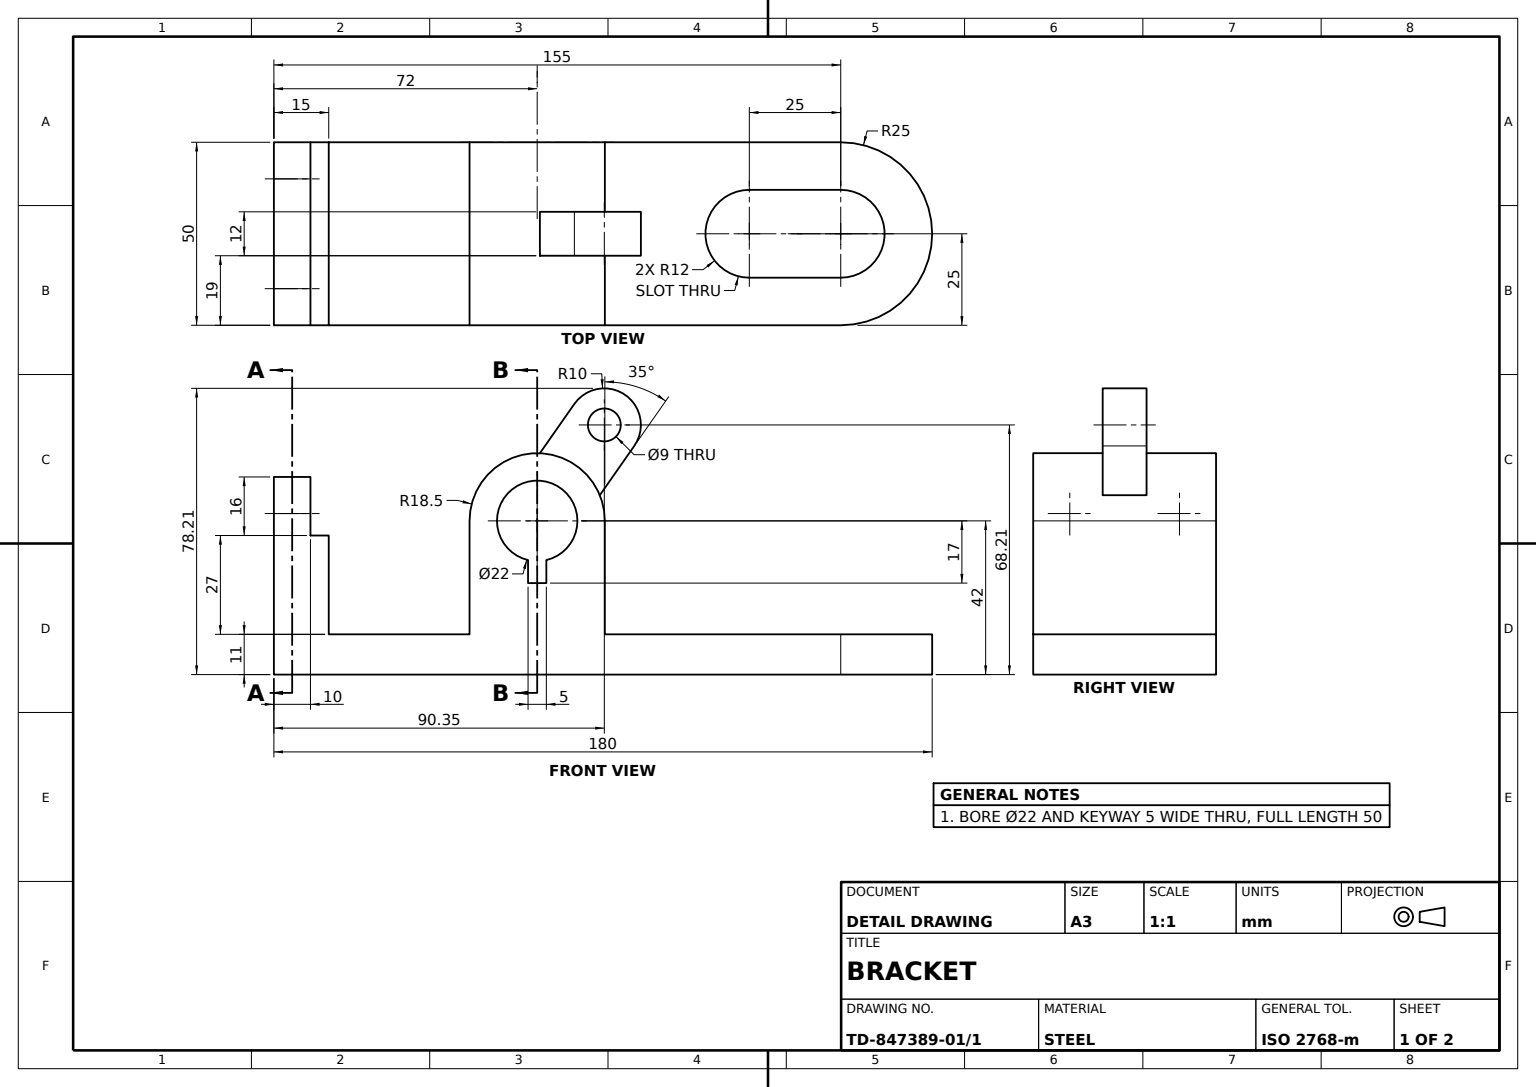
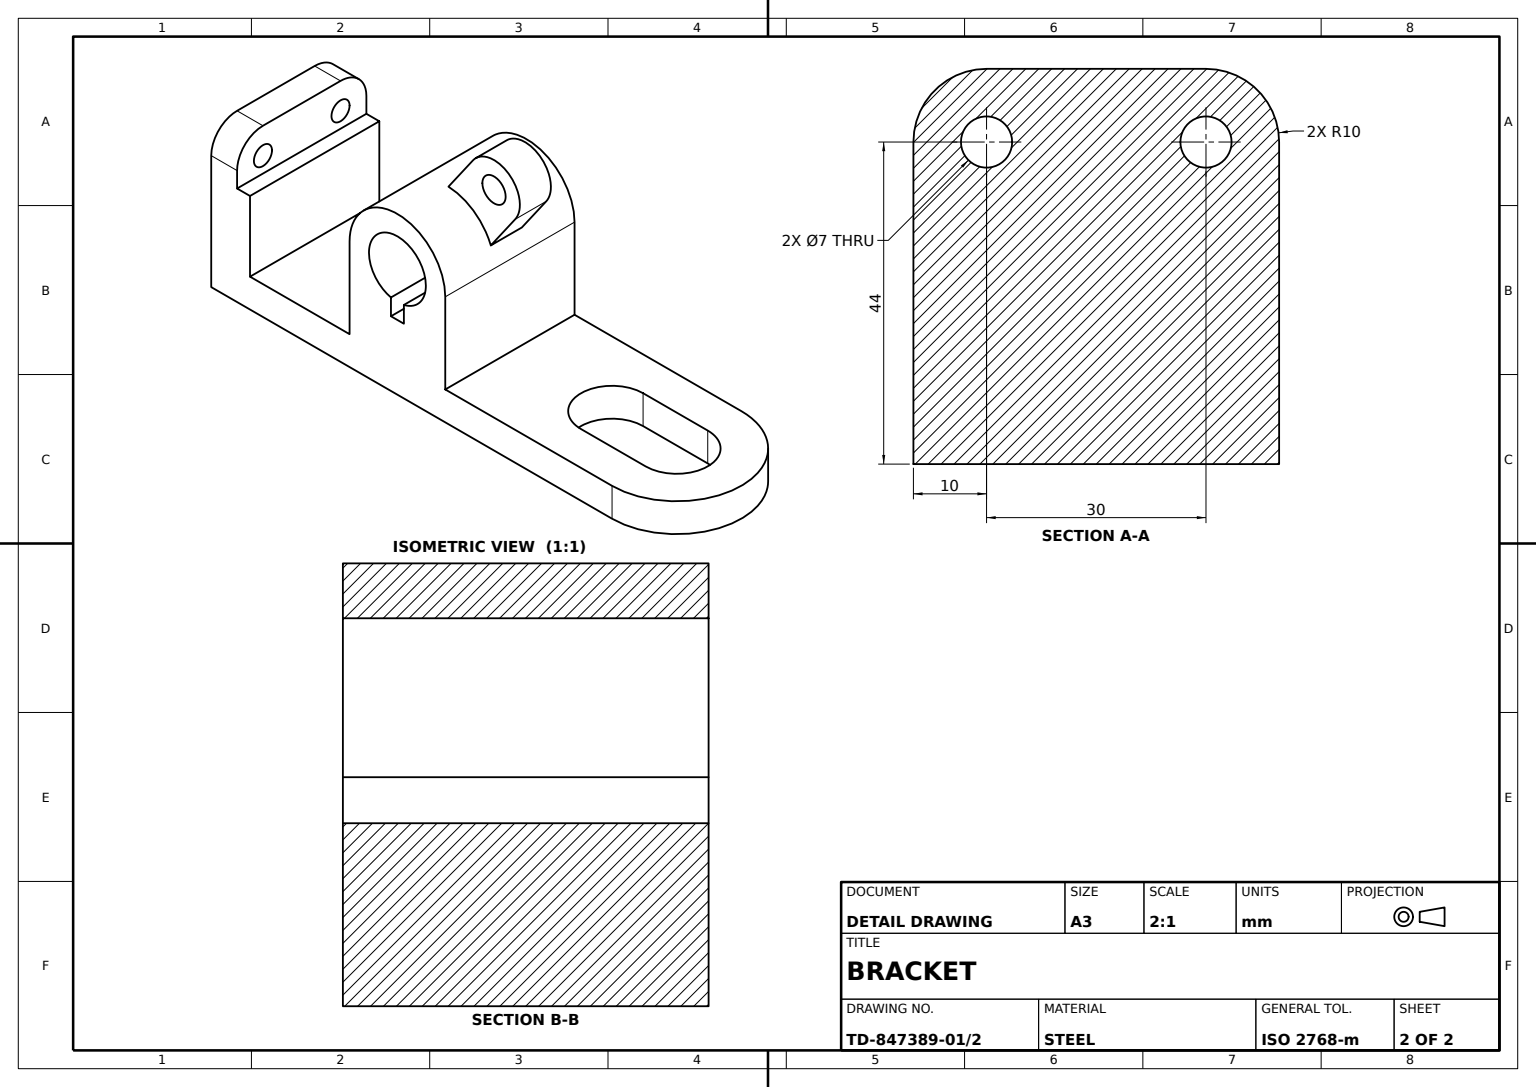
from build123d import *

# Parameters (mm, degrees)
BASE_PLATE_11MM_DEPTH   = 11
CHANNEL_CUT_12X25_DEPTH = 102
BORE_BLOCK_DEPTH        = 50
KEYED_BORE_11_DEPTH     = 68
ANGLED_LUG_DEPTH        = 6
LUG_HOLE_SKETCH_R       = 4.5
LUG_HOLE_9_DEPTH        = 20
END_LUG_SKETCH_W        = 15
END_LUG_SKETCH_H        = 50
END_LUG_DEPTH           = 27
END_LUG_TIP_SKETCH_W    = 10
END_LUG_TIP_SKETCH_H    = 50
END_LUG_TIP_DEPTH       = 16
END_LUG_ROUND_R10_A_R   = 10
END_LUG_ROUND_R10_B_R   = 10
END_LUG_CUT_SKETCH_R    = 3.5
END_LUG_CUT_7_DEPTH     = 16


with BuildPart() as part:
    # Base Plate Sketch → Base Plate 11mm (new body)
    with BuildSketch(Plane(origin=(0, 0, 0), x_dir=(1, 0, 0), z_dir=(0, 1, 0))):
        with BuildLine():
            Line((77.5, -25), (-77.5, -25))
            Line((-77.5, -25), (-77.5, 25))
            Line((-77.5, 25), (77.5, 25))
            ThreePointArc((77.5, 25), (102.5, 0), (77.5, -25))
        make_face()
    extrude(amount=BASE_PLATE_11MM_DEPTH)

    # Channel Cut Sketch → Channel Cut 12x25 (cut)
    with BuildSketch(Plane(origin=(0, 11, 0), x_dir=(1, 0, 0), z_dir=(0, 1, 0))):
        with BuildLine():
            Line((52.5, 12), (77.5, 12))
            ThreePointArc((77.5, 12), (89.5, 0), (77.5, -12))
            Line((77.5, -12), (52.5, -12))
            ThreePointArc((52.5, -12), (40.5, 0), (52.5, 12))
        make_face()
    extrude(amount=-CHANNEL_CUT_12X25_DEPTH, mode=Mode.SUBTRACT)

    # Bore Block Sketch → Bore Block (add)
    with BuildSketch(Plane.XY.offset(25)):
        with BuildLine():
            Line((-24, 11), (13, 11))
            Line((13, 11), (13, 42))
            ThreePointArc((13, 42), (-5.5, 60.5), (-24, 42))
            Line((-24, 42), (-24, 11))
        make_face()
    extrude(amount=-BORE_BLOCK_DEPTH)

    # Keyed Bore Sketch → Keyed Bore Ø11 (cut)
    with BuildSketch(Plane.XY.offset(25)):
        with BuildLine():
            Line((-5.5, 25), (-3, 25))
            Line((-3, 25), (-3, 31.287857357))
            ThreePointArc((-3, 31.287857357), (-5.5, 53), (-8, 31.287857357))
            Line((-8, 31.287857357), (-8, 25))
            Line((-8, 25), (-5.5, 25))
        make_face()
    extrude(amount=-KEYED_BORE_11_DEPTH, mode=Mode.SUBTRACT)

    # Angled Lug Sketch → Angled Lug (add, symmetric)
    with BuildSketch(Plane.XY):
        with BuildLine():
            Line((11.618883443, 49.013831311), (21.045966406, 62.477101054))
            ThreePointArc((21.045966406, 62.477101054), (18.590210327, 76.40438586), (4.66292552, 73.948629781))
            Line((4.66292552, 73.948629781), (-4.764157443, 60.485360038))
            ThreePointArc((-4.764157443, 60.485360038), (5.111164072, 57.154312819), (11.618883443, 49.013831311))
        make_face()
    extrude(amount=ANGLED_LUG_DEPTH, both=True)

    # Lug Hole Sketch → Lug Hole Ø9 (cut)
    with BuildSketch(Plane.XY.offset(6)):
        with Locations((12.854445963, 68.212865417)):
            Circle(LUG_HOLE_SKETCH_R)
    extrude(amount=-LUG_HOLE_9_DEPTH, mode=Mode.SUBTRACT)

    # End Lug Sketch → End Lug (add)
    with BuildSketch(Plane(origin=(0, 11, 0), x_dir=(1, 0, 0), z_dir=(0, 1, 0))):
        with Locations((-70, 0)):
            Rectangle(END_LUG_SKETCH_W, END_LUG_SKETCH_H)
    extrude(amount=END_LUG_DEPTH)

    # End Lug Tip Sketch → End Lug Tip (add)
    with BuildSketch(Plane(origin=(0, 38, 0), x_dir=(1, 0, 0), z_dir=(0, 1, 0))):
        with Locations((-72.5, 0)):
            Rectangle(END_LUG_TIP_SKETCH_W, END_LUG_TIP_SKETCH_H)
    extrude(amount=END_LUG_TIP_DEPTH)

    # End Lug Round R10 A
    end_lug_round_r10_a_edges = [part.edges().sort_by_distance(p)[0] for p in [
        (-72.5, 54, 25),
    ]]
    fillet(end_lug_round_r10_a_edges, radius=END_LUG_ROUND_R10_A_R)

    # End Lug Round R10 B
    end_lug_round_r10_b_edges = [part.edges().sort_by_distance(p)[0] for p in [
        (-72.5, 54, -25),
    ]]
    fillet(end_lug_round_r10_b_edges, radius=END_LUG_ROUND_R10_B_R)

    # End Lug Cut Sketch → End Lug Cut Ø7 (cut)
    with BuildSketch(Plane.ZY.offset(77.5)):
        with Locations((15, 44)):
            Circle(END_LUG_CUT_SKETCH_R)
        with Locations((-15, 44)):
            Circle(END_LUG_CUT_SKETCH_R)
    extrude(amount=-END_LUG_CUT_7_DEPTH, mode=Mode.SUBTRACT)


solid = part.part
